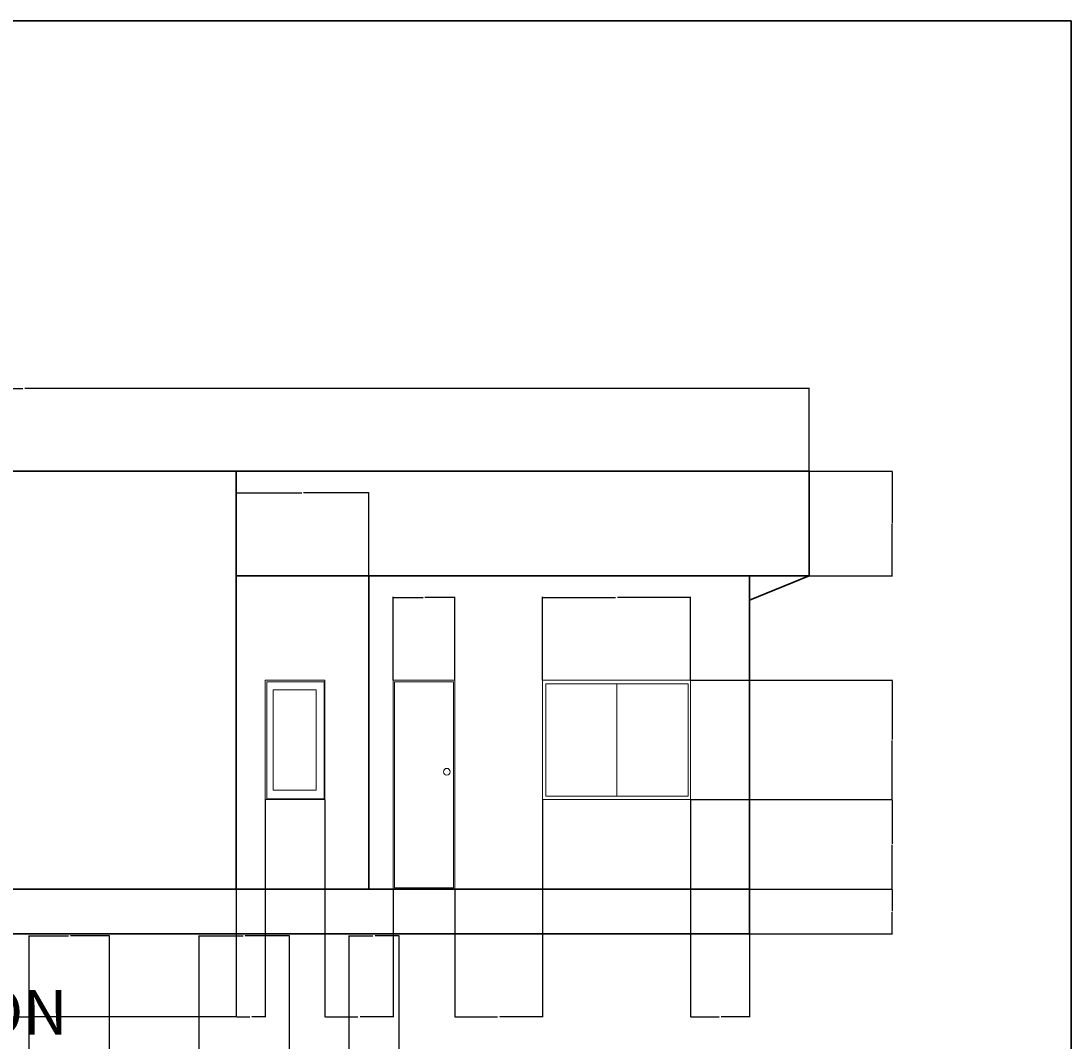
# Model space of a CAD drawing. Units: inches. Extents: x 392 to 1254, y 1207 to 2665.
# Tile 15 of 15: x 832 to 1254, y 2255 to 2665. Entities that reach past the tile are written whole.
import ezdxf

# ---------------------------------------------------------------- set-up
doc = ezdxf.new("R2010")
doc.units = ezdxf.units.IN
for name, color, linetype, lineweight in [('A-ANNO-DIMS', 2, 'Continuous', 18), ('A-ANNO-TEXT', 7, 'Continuous', 25), ('A-ANNO-TTLB', 7, 'Continuous', 35), ('A-ELEV', 7, 'Continuous', 35), ('A-ELEV-OPEN', 4, 'Continuous', 18)]:
    doc.layers.add(name, color=color, linetype=linetype, lineweight=lineweight)
doc.styles.get("Standard").update_dxf_attribs({"font": 'arial.ttf'})
doc.dimstyles.get("Standard").update_dxf_attribs({"dimtxt": 0.18, "dimasz": 0.18, "dimexe": 0.18, "dimexo": 0.0625, "dimgap": 0.09, "dimtad": 0, "dimtih": 1, "dimtoh": 1, "dimdec": 4, "dimzin": 0, "dimdsep": 46, "dimtxsty": 'Standard', "dimcen": 0.09, "dimadec": 0, "dimazin": 0, "dimtfac": 1, "dimtdec": 4, "dimtofl": 0, "dimtmove": 0, "dimatfit": 3, "dimfxl": 1, "dimtolj": 1, "dimtzin": 0, "dimarcsym": 0})

# ---------------------------------------------------------------- blocks, each defined once
blk = doc.blocks.new('*D47')
at = {"layer": 'A-ANNO-DIMS', "color": 0, "lineweight": -2, "transparency": 16777216}
for p, q in [((903.51, 2229.36), (903.51, 2297.33)), ((903.69, 2297.15), (921.29, 2297.15)), ((939.68, 2297.15), (922.08, 2297.15)), ((939.86, 2229.36), (939.86, 2297.33))]:
    blk.add_line(p, q, dxfattribs=at)
at = {"layer": 'A-ANNO-DIMS', "color": 0, "transparency": 16777216}
for points in [[(903.69, 2297.18), (903.69, 2297.12), (903.51, 2297.15)], [(939.68, 2297.18), (939.68, 2297.12), (939.86, 2297.15)]]:
    blk.add_solid(points, dxfattribs=at)
at = {"layer": 'Defpoints', "color": 0, "transparency": 16777216}
for p in [(939.86, 2297.15), (903.51, 2229.3), (939.86, 2229.3)]:
    blk.add_point(p, dxfattribs=at)
at = {"layer": 'A-ANNO-DIMS', "color": 0, "transparency": 16777216, "insert": (921.68, 2297.15), "char_height": 0.18, "attachment_point": 5}
blk.add_mtext('\\A1;36.35', dxfattribs=at)
blk = doc.blocks.new('*D48')
at = {"layer": 'A-ANNO-DIMS', "color": 0, "lineweight": -2, "transparency": 16777216}
for p, q in [((963.86, 2229.36), (963.86, 2297.33)), ((964.04, 2297.15), (973.41, 2297.15)), ((983.71, 2297.15), (974.34, 2297.15)), ((983.89, 2229.36), (983.89, 2297.33))]:
    blk.add_line(p, q, dxfattribs=at)
at = {"layer": 'A-ANNO-DIMS', "color": 0, "transparency": 16777216}
for points in [[(964.04, 2297.18), (964.04, 2297.12), (963.86, 2297.15)], [(983.71, 2297.18), (983.71, 2297.12), (983.89, 2297.15)]]:
    blk.add_solid(points, dxfattribs=at)
at = {"layer": 'Defpoints', "color": 0, "transparency": 16777216}
for p in [(983.89, 2297.15), (963.86, 2229.3), (983.89, 2229.3)]:
    blk.add_point(p, dxfattribs=at)
at = {"layer": 'A-ANNO-DIMS', "color": 0, "transparency": 16777216, "insert": (973.87, 2297.15), "char_height": 0.18, "attachment_point": 5}
blk.add_mtext('\\A1;20.026', dxfattribs=at)
blk = doc.blocks.new('*D49')
at = {"layer": 'A-ANNO-DIMS', "color": 0, "lineweight": -2, "transparency": 16777216}
for p, q in [((835.28, 2224.86), (835.28, 2297.33)), ((835.46, 2297.15), (851, 2297.15)), ((867.33, 2297.15), (851.79, 2297.15)), ((867.51, 2224.86), (867.51, 2297.33))]:
    blk.add_line(p, q, dxfattribs=at)
at = {"layer": 'A-ANNO-DIMS', "color": 0, "transparency": 16777216}
for points in [[(835.46, 2297.18), (835.46, 2297.12), (835.28, 2297.15)], [(867.33, 2297.18), (867.33, 2297.12), (867.51, 2297.15)]]:
    blk.add_solid(points, dxfattribs=at)
at = {"layer": 'Defpoints', "color": 0, "transparency": 16777216}
for p in [(867.51, 2297.15), (835.28, 2224.8), (867.51, 2224.8)]:
    blk.add_point(p, dxfattribs=at)
at = {"layer": 'A-ANNO-DIMS', "color": 0, "transparency": 16777216, "insert": (851.39, 2297.15), "char_height": 0.18, "attachment_point": 5}
blk.add_mtext('\\A1;32.23', dxfattribs=at)
blk = doc.blocks.new('*D54')
at = {"layer": 'A-ANNO-DIMS', "color": 0, "lineweight": -2, "transparency": 16777216}
for p, q in [((517.28, 2483.97), (517.28, 2517.38)), ((517.46, 2517.2), (832.64, 2517.2)), ((1148.6, 2517.2), (833.43, 2517.2)), ((1148.78, 2483.97), (1148.78, 2517.38))]:
    blk.add_line(p, q, dxfattribs=at)
at = {"layer": 'A-ANNO-DIMS', "color": 0, "transparency": 16777216}
for points in [[(517.46, 2517.23), (517.46, 2517.17), (517.28, 2517.2)], [(1148.6, 2517.23), (1148.6, 2517.17), (1148.78, 2517.2)]]:
    blk.add_solid(points, dxfattribs=at)
at = {"layer": 'Defpoints', "color": 0, "transparency": 16777216}
for p in [(1148.78, 2517.2), (517.28, 2483.9), (1148.78, 2483.9)]:
    blk.add_point(p, dxfattribs=at)
at = {"layer": 'A-ANNO-DIMS', "color": 0, "transparency": 16777216, "insert": (833.03, 2517.2), "char_height": 0.18, "attachment_point": 5}
blk.add_mtext('\\A1;631.5', dxfattribs=at)
blk = doc.blocks.new('*D56')
at = {"layer": 'A-ANNO-DIMS', "color": 0, "lineweight": -2, "transparency": 16777216}
for p, q in [((1124.84, 2315.9), (1182.26, 2315.9)), ((1182.08, 2315.72), (1182.08, 2307.08)), ((1182.08, 2298.08), (1182.08, 2306.72)), ((1124.84, 2297.9), (1182.26, 2297.9))]:
    blk.add_line(p, q, dxfattribs=at)
at = {"layer": 'A-ANNO-DIMS', "color": 0, "transparency": 16777216}
for points in [[(1182.05, 2315.72), (1182.11, 2315.72), (1182.08, 2315.9)], [(1182.05, 2298.08), (1182.11, 2298.08), (1182.08, 2297.9)]]:
    blk.add_solid(points, dxfattribs=at)
at = {"layer": 'Defpoints', "color": 0, "transparency": 16777216}
for p in [(1124.78, 2315.9), (1182.08, 2315.9), (1124.78, 2297.9)]:
    blk.add_point(p, dxfattribs=at)
at = {"layer": 'A-ANNO-DIMS', "color": 0, "transparency": 16777216, "insert": (1182.08, 2306.9), "char_height": 0.18, "attachment_point": 5}
blk.add_mtext('\\A1;18', dxfattribs=at)
blk = doc.blocks.new('*D57')
at = {"layer": 'A-ANNO-DIMS', "color": 0, "lineweight": -2, "transparency": 16777216}
for p, q in [((1148.84, 2483.9), (1182.26, 2483.9)), ((1182.08, 2483.72), (1182.08, 2463.08)), ((1182.08, 2442.08), (1182.08, 2462.72)), ((1148.84, 2441.9), (1182.26, 2441.9))]:
    blk.add_line(p, q, dxfattribs=at)
at = {"layer": 'A-ANNO-DIMS', "color": 0, "transparency": 16777216}
for points in [[(1182.05, 2483.72), (1182.11, 2483.72), (1182.08, 2483.9)], [(1182.05, 2442.08), (1182.11, 2442.08), (1182.08, 2441.9)]]:
    blk.add_solid(points, dxfattribs=at)
at = {"layer": 'Defpoints', "color": 0, "transparency": 16777216}
for p in [(1148.78, 2483.9), (1182.08, 2483.9), (1148.78, 2441.9)]:
    blk.add_point(p, dxfattribs=at)
at = {"layer": 'A-ANNO-DIMS', "color": 0, "transparency": 16777216, "insert": (1182.08, 2462.9), "char_height": 0.18, "attachment_point": 5}
blk.add_mtext('\\A1;42', dxfattribs=at)
blk = doc.blocks.new('*D58')
at = {"layer": 'A-ANNO-DIMS', "color": 0, "lineweight": -2, "transparency": 16777216}
for p, q in [((1101.13, 2399.9), (1182.26, 2399.9)), ((1182.08, 2399.72), (1182.08, 2376.08)), ((1182.08, 2352.08), (1182.08, 2375.72)), ((1101.13, 2351.9), (1182.26, 2351.9))]:
    blk.add_line(p, q, dxfattribs=at)
at = {"layer": 'A-ANNO-DIMS', "color": 0, "transparency": 16777216}
for points in [[(1182.05, 2399.72), (1182.11, 2399.72), (1182.08, 2399.9)], [(1182.05, 2352.08), (1182.11, 2352.08), (1182.08, 2351.9)]]:
    blk.add_solid(points, dxfattribs=at)
at = {"layer": 'Defpoints', "color": 0, "transparency": 16777216}
for p in [(1101.07, 2399.9), (1182.08, 2399.9), (1101.07, 2351.9)]:
    blk.add_point(p, dxfattribs=at)
at = {"layer": 'A-ANNO-DIMS', "color": 0, "transparency": 16777216, "insert": (1182.08, 2375.9), "char_height": 0.18, "attachment_point": 5}
blk.add_mtext('\\A1;48', dxfattribs=at)
blk = doc.blocks.new('*D59')
at = {"layer": 'A-ANNO-DIMS', "color": 0, "lineweight": -2, "transparency": 16777216}
for p, q in [((1101.13, 2351.9), (1182.26, 2351.9)), ((1182.08, 2351.72), (1182.08, 2334.08)), ((1182.08, 2316.08), (1182.08, 2333.72)), ((1124.84, 2315.9), (1182.26, 2315.9))]:
    blk.add_line(p, q, dxfattribs=at)
at = {"layer": 'A-ANNO-DIMS', "color": 0, "transparency": 16777216}
for points in [[(1182.05, 2351.72), (1182.11, 2351.72), (1182.08, 2351.9)], [(1182.05, 2316.08), (1182.11, 2316.08), (1182.08, 2315.9)]]:
    blk.add_solid(points, dxfattribs=at)
at = {"layer": 'Defpoints', "color": 0, "transparency": 16777216}
for p in [(1101.07, 2351.9), (1182.08, 2351.9), (1124.78, 2315.9)]:
    blk.add_point(p, dxfattribs=at)
at = {"layer": 'A-ANNO-DIMS', "color": 0, "transparency": 16777216, "insert": (1182.08, 2333.9), "char_height": 0.18, "attachment_point": 5}
blk.add_mtext('\\A1;36', dxfattribs=at)
blk = doc.blocks.new('*D62')
at = {"layer": 'A-ANNO-DIMS', "color": 0, "lineweight": -2, "transparency": 16777216}
for p, q in [((918.49, 2441.97), (918.49, 2475.38)), ((918.67, 2475.2), (944.81, 2475.2)), ((971.6, 2475.2), (945.46, 2475.2)), ((971.78, 2441.97), (971.78, 2475.38))]:
    blk.add_line(p, q, dxfattribs=at)
at = {"layer": 'A-ANNO-DIMS', "color": 0, "transparency": 16777216}
for points in [[(918.67, 2475.23), (918.67, 2475.17), (918.49, 2475.2)], [(971.6, 2475.23), (971.6, 2475.17), (971.78, 2475.2)]]:
    blk.add_solid(points, dxfattribs=at)
at = {"layer": 'Defpoints', "color": 0, "transparency": 16777216}
for p in [(971.78, 2475.2), (918.49, 2441.9), (971.78, 2441.9)]:
    blk.add_point(p, dxfattribs=at)
at = {"layer": 'A-ANNO-DIMS', "color": 0, "transparency": 16777216, "insert": (945.13, 2475.2), "char_height": 0.18, "attachment_point": 5}
blk.add_mtext('\\A1;53.3', dxfattribs=at)
blk = doc.blocks.new('*D68')
at = {"layer": 'A-ANNO-DIMS', "color": 0, "lineweight": -2, "transparency": 16777216}
for p, q in [((753.29, 2315.84), (753.29, 2264.42)), ((918.49, 2315.84), (918.49, 2264.42)), ((753.47, 2264.6), (835.5, 2264.6)), ((918.31, 2264.6), (836.27, 2264.6))]:
    blk.add_line(p, q, dxfattribs=at)
at = {"layer": 'A-ANNO-DIMS', "color": 0, "transparency": 16777216}
for points in [[(753.47, 2264.63), (753.47, 2264.57), (753.29, 2264.6)], [(918.31, 2264.63), (918.31, 2264.57), (918.49, 2264.6)]]:
    blk.add_solid(points, dxfattribs=at)
at = {"layer": 'Defpoints', "color": 0, "transparency": 16777216}
for p in [(753.29, 2315.9), (918.49, 2315.9), (918.49, 2264.6)]:
    blk.add_point(p, dxfattribs=at)
at = {"layer": 'A-ANNO-DIMS', "color": 0, "transparency": 16777216, "insert": (835.89, 2264.6), "char_height": 0.18, "attachment_point": 5}
blk.add_mtext('\\A1;165.2', dxfattribs=at)
blk = doc.blocks.new('*D69')
at = {"layer": 'A-ANNO-DIMS', "color": 0, "lineweight": -2, "transparency": 16777216}
for p, q in [((930.12, 2351.84), (930.12, 2264.42)), ((918.49, 2315.84), (918.49, 2264.42)), ((918.67, 2264.6), (923.92, 2264.6)), ((929.94, 2264.6), (924.69, 2264.6))]:
    blk.add_line(p, q, dxfattribs=at)
at = {"layer": 'A-ANNO-DIMS', "color": 0, "transparency": 16777216}
for points in [[(918.67, 2264.63), (918.67, 2264.57), (918.49, 2264.6)], [(929.94, 2264.63), (929.94, 2264.57), (930.12, 2264.6)]]:
    blk.add_solid(points, dxfattribs=at)
at = {"layer": 'Defpoints', "color": 0, "transparency": 16777216}
for p in [(930.12, 2351.9), (918.49, 2315.9), (930.12, 2264.6)]:
    blk.add_point(p, dxfattribs=at)
at = {"layer": 'A-ANNO-DIMS', "color": 0, "transparency": 16777216, "insert": (924.31, 2264.6), "char_height": 0.18, "attachment_point": 5}
blk.add_mtext('\\A1;11.64', dxfattribs=at)
blk = doc.blocks.new('*D70')
at = {"layer": 'A-ANNO-DIMS', "color": 0, "lineweight": -2, "transparency": 16777216}
for p, q in [((954.12, 2351.84), (954.12, 2264.42)), ((981.57, 2315.84), (981.57, 2264.42)), ((954.3, 2264.6), (967.38, 2264.6)), ((981.39, 2264.6), (968.31, 2264.6))]:
    blk.add_line(p, q, dxfattribs=at)
at = {"layer": 'A-ANNO-DIMS', "color": 0, "transparency": 16777216}
for points in [[(954.3, 2264.63), (954.3, 2264.57), (954.12, 2264.6)], [(981.39, 2264.63), (981.39, 2264.57), (981.57, 2264.6)]]:
    blk.add_solid(points, dxfattribs=at)
at = {"layer": 'Defpoints', "color": 0, "transparency": 16777216}
for p in [(954.12, 2351.9), (981.57, 2315.9), (981.57, 2264.6)]:
    blk.add_point(p, dxfattribs=at)
at = {"layer": 'A-ANNO-DIMS', "color": 0, "transparency": 16777216, "insert": (967.85, 2264.6), "char_height": 0.18, "attachment_point": 5}
blk.add_mtext('\\A1;27.447', dxfattribs=at)
blk = doc.blocks.new('*D71')
at = {"layer": 'A-ANNO-DIMS', "color": 0, "lineweight": -2, "transparency": 16777216}
for p, q in [((981.57, 2399.97), (981.57, 2433.38)), ((981.75, 2433.2), (993.55, 2433.2)), ((1006.1, 2433.2), (994.3, 2433.2)), ((1006.28, 2399.97), (1006.28, 2433.38))]:
    blk.add_line(p, q, dxfattribs=at)
at = {"layer": 'A-ANNO-DIMS', "color": 0, "transparency": 16777216}
for points in [[(981.75, 2433.23), (981.75, 2433.17), (981.57, 2433.2)], [(1006.1, 2433.23), (1006.1, 2433.17), (1006.28, 2433.2)]]:
    blk.add_solid(points, dxfattribs=at)
at = {"layer": 'Defpoints', "color": 0, "transparency": 16777216}
for p in [(1006.28, 2433.2), (981.57, 2399.9), (1006.28, 2399.9)]:
    blk.add_point(p, dxfattribs=at)
at = {"layer": 'A-ANNO-DIMS', "color": 0, "transparency": 16777216, "insert": (993.93, 2433.2), "char_height": 0.18, "attachment_point": 5}
blk.add_mtext('\\A1;24.71', dxfattribs=at)
blk = doc.blocks.new('*D72')
at = {"layer": 'A-ANNO-DIMS', "color": 0, "lineweight": -2, "transparency": 16777216}
for p, q in [((1041.61, 2351.84), (1041.61, 2264.42)), ((1006.28, 2315.84), (1006.28, 2264.42)), ((1006.46, 2264.6), (1023.48, 2264.6)), ((1041.43, 2264.6), (1024.41, 2264.6))]:
    blk.add_line(p, q, dxfattribs=at)
at = {"layer": 'A-ANNO-DIMS', "color": 0, "transparency": 16777216}
for points in [[(1006.46, 2264.63), (1006.46, 2264.57), (1006.28, 2264.6)], [(1041.43, 2264.63), (1041.43, 2264.57), (1041.61, 2264.6)]]:
    blk.add_solid(points, dxfattribs=at)
at = {"layer": 'Defpoints', "color": 0, "transparency": 16777216}
for p in [(1041.61, 2351.9), (1006.28, 2315.9), (1041.61, 2264.6)]:
    blk.add_point(p, dxfattribs=at)
at = {"layer": 'A-ANNO-DIMS', "color": 0, "transparency": 16777216, "insert": (1023.94, 2264.6), "char_height": 0.18, "attachment_point": 5}
blk.add_mtext('\\A1;35.326', dxfattribs=at)
blk = doc.blocks.new('*D73')
at = {"layer": 'A-ANNO-DIMS', "color": 0, "lineweight": -2, "transparency": 16777216}
for p, q in [((1041.61, 2399.97), (1041.61, 2433.38)), ((1041.79, 2433.2), (1070.94, 2433.2)), ((1100.89, 2433.2), (1071.73, 2433.2)), ((1101.07, 2399.97), (1101.07, 2433.38))]:
    blk.add_line(p, q, dxfattribs=at)
at = {"layer": 'A-ANNO-DIMS', "color": 0, "transparency": 16777216}
for points in [[(1041.79, 2433.23), (1041.79, 2433.17), (1041.61, 2433.2)], [(1100.89, 2433.23), (1100.89, 2433.17), (1101.07, 2433.2)]]:
    blk.add_solid(points, dxfattribs=at)
at = {"layer": 'Defpoints', "color": 0, "transparency": 16777216}
for p in [(1101.07, 2433.2), (1041.61, 2399.9), (1101.07, 2399.9)]:
    blk.add_point(p, dxfattribs=at)
at = {"layer": 'A-ANNO-DIMS', "color": 0, "transparency": 16777216, "insert": (1071.34, 2433.2), "char_height": 0.18, "attachment_point": 5}
blk.add_mtext('\\A1;59.46', dxfattribs=at)
blk = doc.blocks.new('*D74')
at = {"layer": 'A-ANNO-DIMS', "color": 0, "lineweight": -2, "transparency": 16777216}
for p, q in [((1101.07, 2351.84), (1101.07, 2264.42)), ((1124.78, 2297.84), (1124.78, 2264.42)), ((1101.25, 2264.6), (1112.55, 2264.6)), ((1124.6, 2264.6), (1113.3, 2264.6))]:
    blk.add_line(p, q, dxfattribs=at)
at = {"layer": 'A-ANNO-DIMS', "color": 0, "transparency": 16777216}
for points in [[(1101.25, 2264.63), (1101.25, 2264.57), (1101.07, 2264.6)], [(1124.6, 2264.63), (1124.6, 2264.57), (1124.78, 2264.6)]]:
    blk.add_solid(points, dxfattribs=at)
at = {"layer": 'Defpoints', "color": 0, "transparency": 16777216}
for p in [(1101.07, 2351.9), (1124.78, 2297.9), (1124.78, 2264.6)]:
    blk.add_point(p, dxfattribs=at)
at = {"layer": 'A-ANNO-DIMS', "color": 0, "transparency": 16777216, "insert": (1112.93, 2264.6), "char_height": 0.18, "attachment_point": 5}
blk.add_mtext('\\A1;23.71', dxfattribs=at)

msp = doc.modelspace()

# ---------------------------------------------------------------- linework, layer by layer
at = {"layer": 'A-ANNO-TTLB'}
msp.add_lwpolyline([(391.939, 2664.8979), (1253.97, 2664.8979), (1253.97, 1207.2611), (391.939, 1207.2611)], close=True, dxfattribs=at)
at = {"layer": 'A-ELEV'}
for p, q in [((1148.7807, 2483.9029), (517.2807, 2483.9029)), ((918.4852, 2441.9029), (918.4852, 2483.9029)), ((1148.7807, 2441.9029), (1148.7807, 2483.9029)), ((1148.7807, 2441.9029), (918.4852, 2441.9029)), ((918.4852, 2435.9029), (918.4852, 2441.9029)), ((971.7807, 2441.9029), (971.7807, 2315.9029)), ((1124.7807, 2441.9029), (1124.7807, 2297.9029)), ((1148.7807, 2441.9029), (1124.7807, 2432.0961)), ((918.4852, 2435.9029), (918.4852, 2315.9029)), ((1124.7807, 2315.9029), (541.2807, 2315.9029)), ((1124.7807, 2297.9029), (541.2807, 2297.9029))]:
    msp.add_line(p, q, dxfattribs=at)
at = {"layer": 'A-ELEV-OPEN'}
for p, q in [((930.1249, 2399.9029), (930.1249, 2351.9029)), ((954.1249, 2399.9029), (930.1249, 2399.9029)), ((954.1249, 2399.9029), (954.1249, 2351.9029)), ((981.5717, 2399.9029), (981.5717, 2315.9029)), ((1006.2807, 2399.9029), (981.5717, 2399.9029)), ((1006.2807, 2399.9029), (1006.2807, 2315.9029)), ((1041.6062, 2399.9029), (1041.6062, 2351.9029)), ((1101.07, 2399.9029), (1041.6062, 2399.9029)), ((1071.4934, 2398.462), (1071.4934, 2353.3573)), ((1101.07, 2399.9029), (1101.07, 2351.9029)), ((954.1249, 2351.9029), (930.1249, 2351.9029)), ((1101.07, 2351.9029), (1041.6062, 2351.9029))]:
    msp.add_line(p, q, dxfattribs=at)
for points in [[(930.7331, 2399.1982), (953.7907, 2399.1982), (953.7907, 2352.2052), (930.7331, 2352.2052)], [(982.0201, 2399.3171), (1005.7633, 2399.3171), (1005.7633, 2316.3943), (982.0201, 2316.3943)], [(1042.9453, 2398.462), (1100.0414, 2398.462), (1100.0414, 2353.3573), (1042.9453, 2353.3573)], [(933.3425, 2396.0994), (950.595, 2396.0994), (950.595, 2355.7407), (933.3425, 2355.7407)]]:
    msp.add_lwpolyline(points, close=True, dxfattribs=at)
msp.add_circle((1003.1069, 2363.1179), 1.358, dxfattribs=at)

# ---------------------------------------------------------------- texts
at = {"layer": 'A-ANNO-TEXT', "insert": (721.3964, 2275.4413), "char_height": 18, "attachment_point": 1}
msp.add_mtext_dynamic_manual_height_columns('ELEVATION', width=295.164206, gutter_width=12.5, heights=[0], dxfattribs=at)

# ---------------------------------------------------------------- dimensions: what is measured, and where the dimension line sits
at = {"layer": 'A-ANNO-DIMS'}
for base, p1, p2, override, picture, middle in [((1148.7807, 2517.2029), (517.2807, 2483.9029), (1148.7807, 2483.9029), {"dimdec": 1, "dimlfac": 1, "dimrnd": 0, "dimzin": 0, "dimdsep": 46, "dimlunit": 2}, '*D54', (833.0307, 2517.2029)), ((971.7807, 2475.2029), (918.4852, 2441.9029), (971.7807, 2441.9029), {"dimdec": 1, "dimlfac": 1, "dimrnd": 0, "dimzin": 0, "dimdsep": 46, "dimlunit": 2}, '*D62', (945.133, 2475.2029)), ((1006.2807, 2433.2029), (981.5717, 2399.9029), (1006.2807, 2399.9029), {"dimdec": 2, "dimlfac": 1, "dimrnd": 0, "dimzin": 0, "dimdsep": 46, "dimlunit": 2}, '*D71', (993.9262, 2433.2029)), ((1101.07, 2433.2029), (1041.6062, 2399.9029), (1101.07, 2399.9029), {"dimdec": 2, "dimlfac": 1, "dimrnd": 0, "dimzin": 0, "dimdsep": 46, "dimlunit": 2}, '*D73', (1071.3381, 2433.2029)), ((930.1249, 2264.6029), (918.4852, 2315.9029), (930.1249, 2351.9029), {"dimdec": 2, "dimlfac": 1, "dimrnd": 0, "dimzin": 0, "dimdsep": 46, "dimlunit": 2}, '*D69', (924.305, 2264.6029)), ((981.5717, 2264.6029), (954.1249, 2351.9029), (981.5717, 2315.9029), {"dimdec": 3, "dimlfac": 1, "dimrnd": 0, "dimzin": 0, "dimdsep": 46, "dimlunit": 2}, '*D70', (967.8483, 2264.6029)), ((1041.60624, 2264.60293), (1006.28071, 2315.90293), (1041.60624, 2351.90293), {"dimdec": 3, "dimlfac": 1, "dimrnd": 0, "dimzin": 0, "dimdsep": 46, "dimlunit": 2}, '*D72', (1023.94347, 2264.60293)), ((1124.7807, 2264.6029), (1101.07, 2351.9029), (1124.7807, 2297.9029), {"dimdec": 2, "dimlfac": 1, "dimrnd": 0, "dimzin": 0, "dimdsep": 46, "dimlunit": 2}, '*D74', (1112.9254, 2264.6029)), ((918.4852, 2264.6029), (753.2885, 2315.9029), (918.4852, 2315.9029), {"dimdec": 1, "dimlfac": 1, "dimrnd": 0, "dimzin": 0, "dimdsep": 46, "dimlunit": 2}, '*D68', (835.8869, 2264.6029)), ((867.5089, 2297.1453), (835.2807, 2224.7953), (867.5089, 2224.7953), {"dimdec": 2, "dimlfac": 1, "dimrnd": 0, "dimzin": 0, "dimdsep": 46, "dimlunit": 2}, '*D49', (851.3948, 2297.1453)), ((939.8604, 2297.1453), (903.5089, 2229.2953), (939.8604, 2229.2953), {"dimdec": 2, "dimlfac": 1, "dimrnd": 0, "dimzin": 0, "dimdsep": 46, "dimlunit": 2}, '*D47', (921.6846, 2297.1453)), ((983.88686, 2297.14532), (963.86038, 2229.29532), (983.88686, 2229.29532), {"dimdec": 3, "dimlfac": 1, "dimrnd": 0, "dimzin": 0, "dimdsep": 46, "dimlunit": 2}, '*D48', (973.87362, 2297.14532))]:
    dim = msp.add_linear_dim(base=base, p1=p1, p2=p2, dimstyle='Standard', override=override, dxfattribs=at)
    dim.commit()
    dim.dimension.update_dxf_attribs({"geometry": picture, "text_midpoint": middle})
for base, p1, p2, picture, middle in [((1182.0807, 2483.9029), (1148.7807, 2441.9029), (1148.7807, 2483.9029), '*D57', (1182.0807, 2462.9029)), ((1182.0807, 2399.9029), (1101.07, 2351.9029), (1101.07, 2399.9029), '*D58', (1182.0807, 2375.9029)), ((1182.0807, 2351.9029), (1124.7807, 2315.9029), (1101.07, 2351.9029), '*D59', (1182.0807, 2333.9029)), ((1182.0807, 2315.9029), (1124.7807, 2297.9029), (1124.7807, 2315.9029), '*D56', (1182.0807, 2306.9029))]:
    dim = msp.add_linear_dim(base=base, p1=p1, p2=p2, angle=90, dimstyle='Standard', override={"dimdec": 0, "dimlfac": 1, "dimrnd": 0, "dimzin": 0, "dimdsep": 46, "dimlunit": 2}, dxfattribs=at)
    dim.commit()
    dim.dimension.update_dxf_attribs({"geometry": picture, "text_midpoint": middle})

doc.saveas('drawing.dxf')
